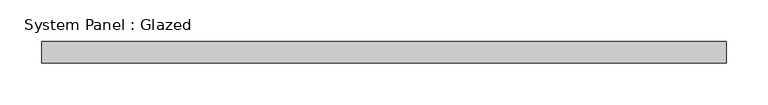
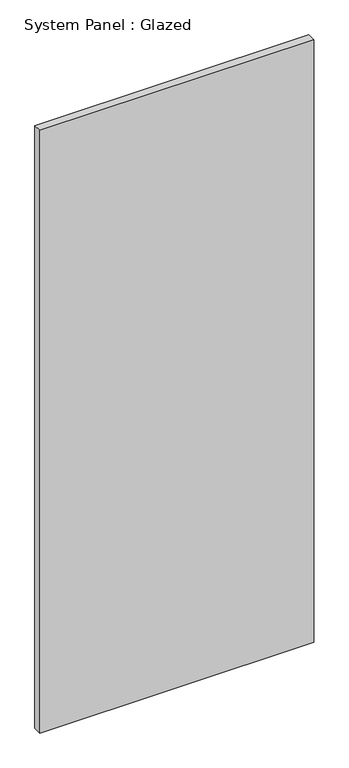
"""IFC4 building model written with IfcOpenShell, lengths in millimetres: plate geometry, System Panel : Glazed."""

from ifc_helpers import new_model, si_unit, origin, origin_with_axes, place, context, project, spatial, polyline, outline, extrude, source, transform, mapped, element, save


def system_panel_glazed_b8cd24f7(model_context):
    return source(origin(), model_context, "Body", "SweptSolid", [
        extrude(outline(polyline([(409.575, 19.05), (-409.575, 19.05), (-409.575, 44.45), (409.575, 44.45), (409.575, 19.05)])), origin_with_axes(), (0.0, 0.0, 1.0), 1905.0),
    ])


if __name__ == "__main__":
    model = new_model("IFC4")
    model_context = context("Model", 3, world=origin())
    ifc_project = project(units=[si_unit("LENGTHUNIT", "METRE", prefix="MILLI")], contexts=[model_context])
    site = spatial("IfcSite", under=ifc_project)
    building = spatial("IfcBuilding", under=site)
    placement = place(None, origin())
    system_panel_glazed_shape = system_panel_glazed_b8cd24f7(model_context)
    element("IfcPlate", 1, ObjectType="System Panel : Glazed", at=placement, inside=building, context=model_context, shape_type="MappedRepresentation", body=[
        mapped(system_panel_glazed_shape, transform((0.0, 0.0, 0.0), x_axis=(1.0, 0.0, 0.0), y_axis=(0.0, 1.0, 0.0), z_axis=(0.0, 0.0, 1.0))),
    ])
    save(model, "model.ifc")

# Revit data of these elements
# Type "System Panel : Glazed"
#   Construction Type Id = "GSP4R"
#   Analytic Construction = "1/8 in Pilkington single glazing"
#   Visual Light Transmittance = 0.9
#   Solar Heat Gain Coefficient = 0.86
#   Heat Transfer Coefficient (U) = 1.18115 BTU/(h·ft²·°F)
#   Define Thermal Properties by = 1
# Element 1 (IfcPlate, "System Panel : Glazed")
#   Materials on its faces: "Glass"
# Materials
#   "Glass": class "Glass", colour RGB 0 128 192, transparency 0.75, Description = "Soda Lime Glass", Cost = 0
